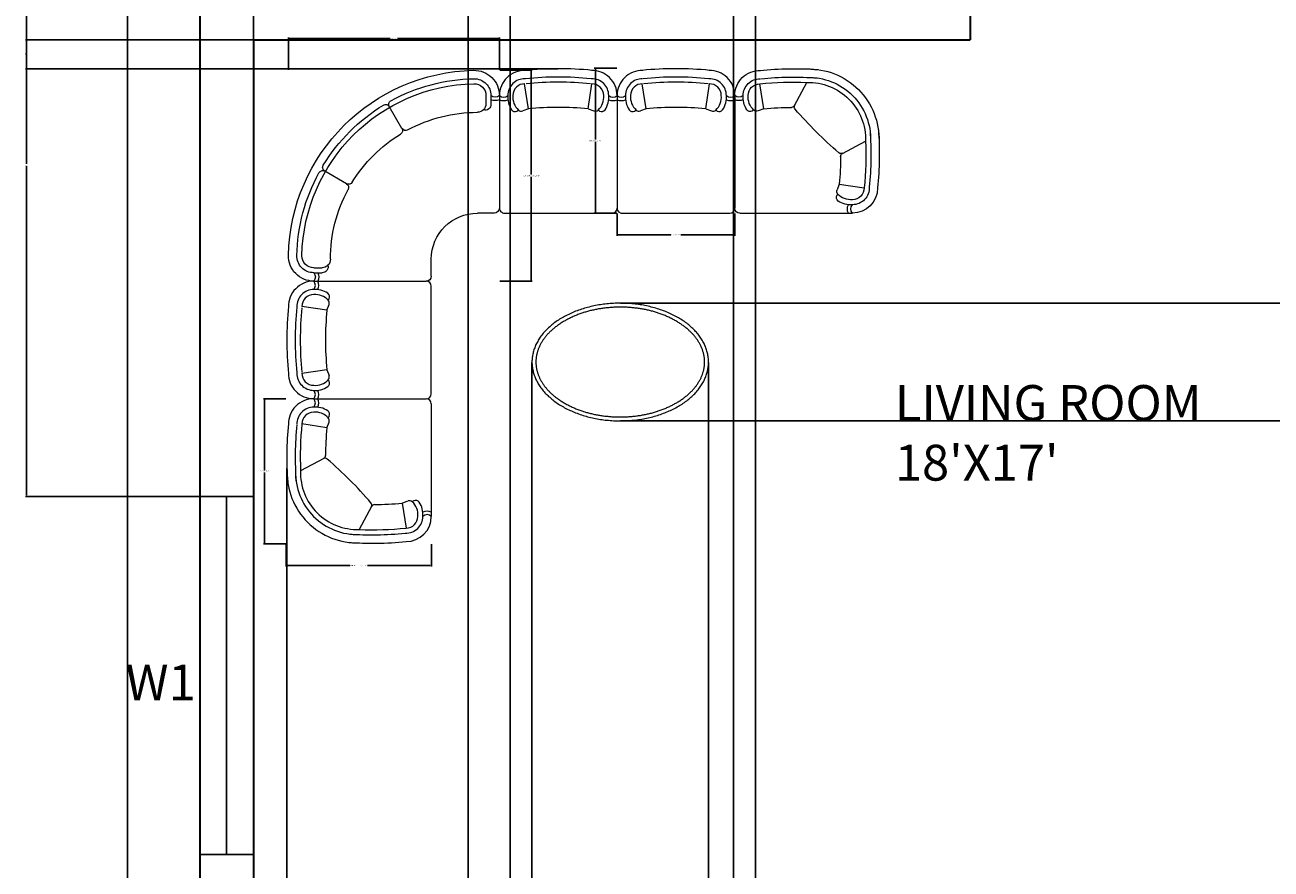
# Model space of a CAD drawing. Units: inches. Extents: x 3 to 420, y -502 to 54.
# Tile 2 of 6: x 3 to 212, y -398 to -257. Entities that reach past the tile are written whole.
import ezdxf

# ---------------------------------------------------------------- set-up
doc = ezdxf.new("R2010")
doc.units = ezdxf.units.IN
doc.header["$MEASUREMENT"] = 0
for name, color, linetype, lineweight in [('A-ANNO-DIMS', 2, 'Continuous', 18), ('A-ANNO-TEXT', 7, 'Continuous', 18), ('A-AREA-IDEN', 7, 'Continuous', 18), ('A-FURN', 8, 'Continuous', 18), ('A-GLAZ', 40, 'Continuous', 25), ('A-WALL', 7, 'Continuous', 35)]:
    doc.layers.add(name, color=color, linetype=linetype, lineweight=lineweight)
doc.styles.get("Standard").update_dxf_attribs({"font": 'arial.ttf'})
doc.dimstyles.get("Standard").update_dxf_attribs({"dimtxt": 0.18, "dimasz": 0.18, "dimexe": 0.18, "dimexo": 0.0625, "dimgap": 0.09, "dimtad": 0, "dimtih": 1, "dimtoh": 1, "dimdec": 0, "dimzin": 0, "dimdsep": 46, "dimlunit": 3, "dimtxsty": 'Standard', "dimcen": 0.09, "dimadec": 0, "dimazin": 0, "dimtfac": 1, "dimtdec": 0, "dimtofl": 0, "dimtmove": 0, "dimatfit": 3, "dimfxl": 1, "dimtolj": 1, "dimtzin": 0, "dimarcsym": 0})

# ---------------------------------------------------------------- blocks, each defined once
blk = doc.blocks.new('*D2')
at = {"layer": 'A-ANNO-DIMS', "color": 0, "lineweight": -2, "transparency": 16777216}
for p, q in [((32.33, 4.54), (20.1, 4.54)), ((20.28, 4.36), (20.28, -230.8)), ((20.28, -472.28), (20.28, -237.11)), ((32.33, -472.46), (20.1, -472.46))]:
    blk.add_line(p, q, dxfattribs=at)
at = {"layer": 'A-ANNO-DIMS', "color": 0, "transparency": 16777216}
for points in [[(20.25, 4.36), (20.31, 4.36), (20.28, 4.54)], [(20.25, -472.28), (20.31, -472.28), (20.28, -472.46)]]:
    blk.add_solid(points, dxfattribs=at)
at = {"layer": 'Defpoints', "color": 0, "transparency": 16777216}
for p in [(32.39, 4.54), (20.28, -472.46), (32.39, -472.46)]:
    blk.add_point(p, dxfattribs=at)
at = {"layer": 'A-ANNO-DIMS', "color": 0, "transparency": 16777216, "insert": (20.28, -233.96), "char_height": 6, "attachment_point": 5}
blk.add_mtext('\\A1;39\'-9"', dxfattribs=at)
blk = doc.blocks.new('A$C707258B2')
at = {"color": 0}
for p, q in [((0.4042, 0.342), (1.0739, 0.342)), ((1.1039, 0.312), (1.1039, 0.212)), ((0.4042, 0.292), (0.4544, 0.292)), ((0.4042, 0.262), (0.4539, 0.262)), ((1.4789, -0.063), (1.3789, -0.063)), ((1.5089, -0.7628), (1.5089, -0.093)), ((0.5998, -0.2378), (0.4699, -0.3128)), ((0.9291, -0.5671), (0.8541, -0.697)), ((1.4289, -0.7628), (1.4289, -0.713)), ((1.4589, -0.7628), (1.4589, -0.7125))]:
    blk.add_line(p, q, dxfattribs=at)
for centre, radius, start, end in [((0.4042, 0.192), 0.15, 90, 181.17538), ((0.3779, 0.317), 0.0362, 316.39718, 43.60282), ((0.3679, 0.317), 0.0662, 337.82984, 22.17016), ((1.0739, 0.312), 0.03, 360, 90), ((0.4042, 0.192), 0.1, 90, 181.17538), ((0.4042, 0.192), 0.07, 90, 181.17538), ((0.4539, 0.212), 0.05, 360, 90), ((0.4548, 0.2564), 0.0357, 345.42616, 90.55549), ((1.3789, 0.212), 1.125, 181.17538, 268.82462), ((1.3789, 0.212), 1.075, 181.17538, 208.63569), ((1.3789, 0.212), 1.045, 181.17538, 268.82462), ((1.3789, 0.212), 0.875, 180, 208.40825), ((1.3789, 0.212), 0.275, 180, 270), ((1.4789, -0.093), 0.03, 360, 90), ((0.5873, -0.2162), 0.025, 300, 28.40825), ((0.6123, -0.2595), 0.025, 31.59175, 120), ((1.3789, 0.212), 0.875, 211.59175, 238.40825), ((0.4574, -0.2912), 0.025, 208.63569, 300), ((0.4824, -0.3345), 0.025, 120, 211.36431), ((1.3789, 0.212), 1.075, 211.36431, 238.63569), ((0.9075, -0.5546), 0.025, 330, 58.40825), ((0.9508, -0.5796), 0.025, 61.59175, 150), ((1.3789, 0.212), 0.875, 241.59175, 270), ((1.3789, -0.713), 0.05, 360, 90), ((0.8324, -0.6845), 0.025, 238.63569, 330), ((0.8757, -0.7095), 0.025, 150, 241.36431), ((1.3789, 0.212), 1.075, 241.36431, 268.82462), ((1.4255, -0.7093), 0.0336, 354.63008, 109.38826), ((1.4839, -0.7988), 0.0662, 67.82984, 112.17016), ((1.3589, -0.7628), 0.15, 268.82462, 360), ((1.3589, -0.7628), 0.1, 268.82462, 360), ((1.3589, -0.7628), 0.07, 268.82462, 360), ((1.4839, -0.789), 0.0362, 46.39718, 133.60282)]:
    blk.add_arc(centre, radius, start, end, dxfattribs=at)
blk = doc.blocks.new('part 01')
at = {"color": 0}
for p, q in [((-669.8, 700), (0, 700)), ((30, 30), (30, 670)), ((-590.9, 527.1), (-739.8, 550)), ((-590.9, 527.1), (-578.5, 561.2)), ((-590.9, 172.9), (-739.8, 150)), ((-590.9, 172.9), (-578.5, 138.8)), ((-669.8, 0), (0, 0))]:
    blk.add_line(p, q, dxfattribs=at)
for centre, radius, start, end in [((-669.8, 550), 150, 90, 181.17538), ((-696, 675), 36.2, 316.39718, 43.60282), ((-705.9, 675), 66.2, 337.82984, 22.17016), ((0, 670), 30, 0, 90), ((-669.8, 550), 100, 90, 181.17538), ((-669.8, 550), 70, 90, 181.17538), ((-659.7, 517.8), 132.7, 56.08973, 95.61316), ((-659.7, 517.8), 102.7, 42.00663, 95.61316), ((-599.7, 607.2), 25, 332.96082, 56.08973), ((-624.8, 620), 53.2, 321.00172, 332.96082), ((1178.1, 350), 2007.9, 174.28354, 185.71646), ((1178.1, 350), 1957.9, 174.28354, 185.71646), ((1178.1, 350), 1927.9, 174.28354, 185.71646), ((1178.1, 350), 1777.9, 174.28354, 185.71646), ((-602, 569.8), 25, 340, 42.00663), ((-669.8, 150), 150, 178.82462, 270), ((-669.8, 150), 100, 178.82462, 270), ((-669.8, 150), 70, 178.82462, 270), ((-659.7, 182.2), 102.7, 264.38684, 317.99337), ((-599.7, 92.8), 25, 303.91027, 27.03918), ((-602, 130.2), 25, 317.99337, 20), ((-624.8, 80), 53.2, 27.03918, 38.99828), ((-659.7, 182.2), 132.7, 264.38684, 303.91027), ((-696, 25), 36.2, 316.39718, 43.60282), ((-705.9, 25), 66.2, 337.82984, 22.17016), ((0, 30), 30, 270, 0)]:
    blk.add_arc(centre, radius, start, end, dxfattribs=at)
blk = doc.blocks.new('part02')
at = {"color": 0}
for p, q in [((0, -669.8), (0, 0)), ((30, 30), (699.8, 30)), ((620.9, -142.9), (608.5, -108.8)), ((620.9, -142.9), (769.8, -120)), ((640.4, -325.6), (778.2, -398.9)), ((172.9, -590.9), (138.8, -578.5)), ((172.9, -590.9), (150, -739.8)), ((355.6, -610.4), (428.9, -748.2))]:
    blk.add_line(p, q, dxfattribs=at)
for centre, radius, start, end in [((30, 0), 30, 90, 180), ((726, 5), 56.2, 153.6122, 206.66656), ((726, 5), 36.2, 136.39718, 223.60282), ((699.8, -120), 150, 0, 90), ((629.7, -62.8), 25, 123.91027, 207.03918), ((689.7, -152.2), 102.7, 84.38684, 137.99337), ((689.3, -151.3), 131.7, 85.43775, 123.98866), ((699.5, -120.6), 100.6, 357.50055, 89.85796), ((699.8, -120), 70, 0, 90), ((632, -100.2), 25, 137.99337, 200), ((654.8, -50), 53.2, 207.03918, 218.99828), ((-1148.1, -320), 1777.9, 0.38365, 5.71646), ((-1228.2, -319.5), 2007.9, 357.73494, 5.70316), ((-1148.1, -320), 1957.9, 355.86566, 5.71646), ((-1148.1, -320), 2007.9, 355.81801, 5.71646), ((2219.8, -2189.8), 2454.4, 130.6961, 139.3039), ((632.4, -344.1), 20, 62, 130.6961), ((649.7, -308), 20, 180.38365, 242), ((439.4, -409.4), 418.9, 268.21809, 1.78191), ((439.4, -409.4), 368.9, 268.21809, 1.78191), ((439.4, -409.4), 338.9, 268.21809, 1.78191), ((182.2, -659.7), 132.7, 146.08973, 185.61316), ((92.8, -599.7), 25, 62.96082, 146.08973), ((182.2, -659.7), 102.7, 132.00663, 185.61316), ((80, -624.8), 53.2, 51.00172, 62.96082), ((130.2, -602), 25, 70, 132.00663), ((350, 1178.1), 1777.9, 264.28354, 269.61635), ((374.1, -602.4), 20, 139.3039, 208), ((25, -696), 56.2, 63.33344, 116.3878), ((25, -696), 36.2, 46.39718, 133.60282), ((338, -619.7), 20, 28, 89.61635), ((150, -669.8), 150, 180, 271.17538), ((150, -669.8), 100, 180, 271.17538), ((150, -669.8), 70, 180, 270), ((349.5, 1258.2), 2007.9, 264.29684, 272.26506), ((350, 1178.1), 1957.9, 264.28354, 274.13434), ((350, 1178.1), 2007.9, 264.28354, 274.18199)]:
    blk.add_arc(centre, radius, start, end, dxfattribs=at)
blk = doc.blocks.new('WIN-W1-60')
for p, q in [((0, 9), (60, 9)), ((0, 9), (0, 0)), ((60, 9), (60, 0)), ((0, 4.5), (60, 4.5)), ((0, 0), (60, 0))]:
    blk.add_line(p, q)
blk = doc.blocks.new('*D21')
at = {"layer": 'A-ANNO-DIMS', "color": 0, "lineweight": -2, "transparency": 16777216}
for p, q in [((102.21, -264.22), (98.45, -264.22)), ((98.63, -264.4), (98.63, -276.18)), ((98.63, -288.33), (98.63, -276.55)), ((102.21, -288.51), (98.45, -288.51))]:
    blk.add_line(p, q, dxfattribs=at)
at = {"layer": 'A-ANNO-DIMS', "color": 0, "transparency": 16777216}
for points in [[(98.6, -264.4), (98.66, -264.4), (98.63, -264.22)], [(98.6, -288.33), (98.66, -288.33), (98.63, -288.51)]]:
    blk.add_solid(points, dxfattribs=at)
at = {"layer": 'Defpoints', "color": 0, "transparency": 16777216}
for p in [(102.27, -264.22), (98.63, -288.51), (102.27, -288.51)]:
    blk.add_point(p, dxfattribs=at)
at = {"layer": 'A-ANNO-DIMS', "color": 0, "transparency": 16777216, "insert": (98.63, -276.37), "char_height": 0.18, "attachment_point": 5}
blk.add_mtext('\\A1;SEAT 2\'-0 1/2" TYP.', dxfattribs=at)
blk = doc.blocks.new('*D22')
at = {"layer": 'A-ANNO-DIMS', "color": 0, "lineweight": -2, "transparency": 16777216}
for p, q in [((102.27, -288.57), (102.27, -292.34)), ((121.97, -288.57), (121.97, -292.34)), ((102.45, -292.16), (111.28, -292.16)), ((121.79, -292.16), (112.96, -292.16))]:
    blk.add_line(p, q, dxfattribs=at)
at = {"layer": 'A-ANNO-DIMS', "color": 0, "transparency": 16777216}
for points in [[(102.45, -292.13), (102.45, -292.19), (102.27, -292.16)], [(121.79, -292.13), (121.79, -292.19), (121.97, -292.16)]]:
    blk.add_solid(points, dxfattribs=at)
at = {"layer": 'Defpoints', "color": 0, "transparency": 16777216}
for p in [(102.27, -288.51), (121.97, -288.51), (121.97, -292.16)]:
    blk.add_point(p, dxfattribs=at)
at = {"layer": 'A-ANNO-DIMS', "color": 0, "transparency": 16777216, "insert": (112.12, -292.16), "char_height": 0.18, "attachment_point": 5}
blk.add_mtext('\\A1;1\'-7 1/2" TYP.', dxfattribs=at)
blk = doc.blocks.new('*D23')
at = {"layer": 'A-ANNO-DIMS', "color": 0, "lineweight": -2, "transparency": 16777216}
for p, q in [((46.88, -343.96), (46.88, -347.72)), ((71.17, -343.96), (71.17, -347.72)), ((47.06, -347.54), (57.55, -347.54)), ((70.99, -347.54), (60.5, -347.54))]:
    blk.add_line(p, q, dxfattribs=at)
at = {"layer": 'A-ANNO-DIMS', "color": 0, "transparency": 16777216}
for points in [[(47.06, -347.51), (47.06, -347.57), (46.88, -347.54)], [(70.99, -347.51), (70.99, -347.57), (71.17, -347.54)]]:
    blk.add_solid(points, dxfattribs=at)
at = {"layer": 'Defpoints', "color": 0, "transparency": 16777216}
for p in [(46.88, -343.9), (71.17, -343.9), (71.17, -347.54)]:
    blk.add_point(p, dxfattribs=at)
at = {"layer": 'A-ANNO-DIMS', "color": 0, "transparency": 16777216, "insert": (59.02, -347.54), "char_height": 0.18, "attachment_point": 5}
blk.add_mtext('\\A1;END UNIT 2\'-0 1/2" TYP.', dxfattribs=at)
blk = doc.blocks.new('*D24')
at = {"layer": 'A-ANNO-DIMS', "color": 0, "lineweight": -2, "transparency": 16777216}
for p, q in [((46.82, -319.61), (43.06, -319.61)), ((43.24, -319.79), (43.24, -331.57)), ((43.24, -343.72), (43.24, -331.94)), ((46.82, -343.9), (43.06, -343.9))]:
    blk.add_line(p, q, dxfattribs=at)
at = {"layer": 'A-ANNO-DIMS', "color": 0, "transparency": 16777216}
for points in [[(43.21, -319.79), (43.27, -319.79), (43.24, -319.61)], [(43.21, -343.72), (43.27, -343.72), (43.24, -343.9)]]:
    blk.add_solid(points, dxfattribs=at)
at = {"layer": 'Defpoints', "color": 0, "transparency": 16777216}
for p in [(46.88, -319.61), (43.24, -343.9), (46.88, -343.9)]:
    blk.add_point(p, dxfattribs=at)
at = {"layer": 'A-ANNO-DIMS', "color": 0, "transparency": 16777216, "insert": (43.24, -331.76), "char_height": 0.18, "attachment_point": 5}
blk.add_mtext('\\A1;2\'-0 1/2" TYP.', dxfattribs=at)
blk = doc.blocks.new('*D25')
at = {"layer": 'A-ANNO-DIMS', "color": 0, "lineweight": -2, "transparency": 16777216}
for p, q in [((82.63, -264.57), (88.05, -264.57)), ((87.87, -264.75), (87.87, -282.06)), ((87.87, -299.73), (87.87, -282.42)), ((82.63, -299.91), (88.05, -299.91))]:
    blk.add_line(p, q, dxfattribs=at)
at = {"layer": 'A-ANNO-DIMS', "color": 0, "transparency": 16777216}
for points in [[(87.84, -264.75), (87.9, -264.75), (87.87, -264.57)], [(87.84, -299.73), (87.9, -299.73), (87.87, -299.91)]]:
    blk.add_solid(points, dxfattribs=at)
at = {"layer": 'Defpoints', "color": 0, "transparency": 16777216}
for p in [(82.57, -264.57), (82.57, -299.91), (87.87, -299.91)]:
    blk.add_point(p, dxfattribs=at)
at = {"layer": 'A-ANNO-DIMS', "color": 0, "transparency": 16777216, "insert": (87.87, -282.24), "char_height": 0.18, "attachment_point": 5}
blk.add_mtext('\\A1;CORNER UNIT 2\'-11 1/2"', dxfattribs=at)
blk = doc.blocks.new('*D26')
at = {"layer": 'A-ANNO-DIMS', "color": 0, "lineweight": -2, "transparency": 16777216}
for p, q in [((47.23, -264.51), (47.23, -259.09)), ((47.41, -259.27), (64.29, -259.27)), ((82.39, -259.27), (65.51, -259.27)), ((82.57, -264.51), (82.57, -259.09))]:
    blk.add_line(p, q, dxfattribs=at)
at = {"layer": 'A-ANNO-DIMS', "color": 0, "transparency": 16777216}
for points in [[(47.41, -259.24), (47.41, -259.3), (47.23, -259.27)], [(82.39, -259.24), (82.39, -259.3), (82.57, -259.27)]]:
    blk.add_solid(points, dxfattribs=at)
at = {"layer": 'Defpoints', "color": 0, "transparency": 16777216}
for p in [(82.57, -259.27), (47.23, -264.57), (82.57, -264.57)]:
    blk.add_point(p, dxfattribs=at)
at = {"layer": 'A-ANNO-DIMS', "color": 0, "transparency": 16777216, "insert": (64.9, -259.27), "char_height": 0.18, "attachment_point": 5}
blk.add_mtext('\\A1;2\'-11 1/2"', dxfattribs=at)
blk = doc.blocks.new('*D39')
at = {"layer": 'A-ANNO-DIMS', "color": 0, "lineweight": -2, "transparency": 16777216}
for p, q in [((41.39, -130.52), (41.39, -501.64)), ((77.36, -130.52), (77.36, -501.64)), ((41.57, -501.46), (59.04, -501.46)), ((77.18, -501.46), (59.7, -501.46))]:
    blk.add_line(p, q, dxfattribs=at)
at = {"layer": 'A-ANNO-DIMS', "color": 0, "transparency": 16777216}
for points in [[(41.57, -501.43), (41.57, -501.49), (41.39, -501.46)], [(77.18, -501.43), (77.18, -501.49), (77.36, -501.46)]]:
    blk.add_solid(points, dxfattribs=at)
at = {"layer": 'Defpoints', "color": 0, "transparency": 16777216}
for p in [(41.39, -130.46), (77.36, -130.46), (77.36, -501.46)]:
    blk.add_point(p, dxfattribs=at)
at = {"layer": 'A-ANNO-DIMS', "color": 0, "transparency": 16777216, "insert": (59.37, -501.46), "char_height": 0.18, "attachment_point": 5}
blk.add_mtext('\\A1;3\'-0"', dxfattribs=at)
blk = doc.blocks.new('*D46')
at = {"layer": 'A-ANNO-DIMS', "color": 0, "lineweight": -2, "transparency": 16777216}
for p, q in [((41.39, -135.02), (41.39, -501.64)), ((121.75, -135.02), (121.75, -501.64)), ((41.57, -501.46), (81.03, -501.46)), ((121.57, -501.46), (82.11, -501.46))]:
    blk.add_line(p, q, dxfattribs=at)
at = {"layer": 'A-ANNO-DIMS', "color": 0, "transparency": 16777216}
for points in [[(41.57, -501.43), (41.57, -501.49), (41.39, -501.46)], [(121.57, -501.43), (121.57, -501.49), (121.75, -501.46)]]:
    blk.add_solid(points, dxfattribs=at)
at = {"layer": 'Defpoints', "color": 0, "transparency": 16777216}
for p in [(41.39, -134.96), (121.75, -134.96), (121.75, -501.46)]:
    blk.add_point(p, dxfattribs=at)
at = {"layer": 'A-ANNO-DIMS', "color": 0, "transparency": 16777216, "insert": (81.57, -501.46), "char_height": 0.18, "attachment_point": 5}
blk.add_mtext('\\A1;6\'-8 1/2"', dxfattribs=at)
blk = doc.blocks.new('*D61')
at = {"layer": 'A-ANNO-DIMS', "color": 0, "lineweight": -2, "transparency": 16777216}
for p, q in [((32.33, -224.96), (3.21, -224.96)), ((3.39, -225.14), (3.39, -280.27)), ((3.39, -335.78), (3.39, -280.64)), ((32.33, -335.96), (3.21, -335.96))]:
    blk.add_line(p, q, dxfattribs=at)
at = {"layer": 'A-ANNO-DIMS', "color": 0, "transparency": 16777216}
for points in [[(3.36, -225.14), (3.42, -225.14), (3.39, -224.96)], [(3.36, -335.78), (3.42, -335.78), (3.39, -335.96)]]:
    blk.add_solid(points, dxfattribs=at)
at = {"layer": 'Defpoints', "color": 0, "transparency": 16777216}
for p in [(32.39, -224.96), (3.39, -335.96), (32.39, -335.96)]:
    blk.add_point(p, dxfattribs=at)
at = {"layer": 'A-ANNO-DIMS', "color": 0, "transparency": 16777216, "insert": (3.39, -280.46), "char_height": 0.18, "attachment_point": 5}
blk.add_mtext('\\A1;9\'-3"', dxfattribs=at)
blk = doc.blocks.new('*D62')
at = {"layer": 'A-ANNO-DIMS', "color": 0, "lineweight": -2, "transparency": 16777216}
for p, q in [((84.39, -463.39), (84.39, 33.72)), ((84.57, 33.54), (104.58, 33.54)), ((125.25, 33.54), (105.24, 33.54)), ((125.43, -463.39), (125.43, 33.72))]:
    blk.add_line(p, q, dxfattribs=at)
at = {"layer": 'A-ANNO-DIMS', "color": 0, "transparency": 16777216}
for points in [[(84.57, 33.57), (84.57, 33.51), (84.39, 33.54)], [(125.25, 33.57), (125.25, 33.51), (125.43, 33.54)]]:
    blk.add_solid(points, dxfattribs=at)
at = {"layer": 'Defpoints', "color": 0, "transparency": 16777216}
for p in [(125.43, 33.54), (84.39, -463.46), (125.43, -463.46)]:
    blk.add_point(p, dxfattribs=at)
at = {"layer": 'A-ANNO-DIMS', "color": 0, "transparency": 16777216, "insert": (104.91, 33.54), "char_height": 0.18, "attachment_point": 5}
blk.add_mtext('\\A1;3\'-5"', dxfattribs=at)
blk = doc.blocks.new('*D73')
at = {"layer": 'A-ANNO-DIMS', "color": 0, "lineweight": -2, "transparency": 16777216}
for p, q in [((88.02, -313.52), (88.02, -501.64)), ((117.58, -313.52), (117.58, -501.64)), ((88.2, -501.46), (102.26, -501.46)), ((117.4, -501.46), (103.34, -501.46))]:
    blk.add_line(p, q, dxfattribs=at)
at = {"layer": 'A-ANNO-DIMS', "color": 0, "transparency": 16777216}
for points in [[(88.2, -501.43), (88.2, -501.49), (88.02, -501.46)], [(117.4, -501.43), (117.4, -501.49), (117.58, -501.46)]]:
    blk.add_solid(points, dxfattribs=at)
at = {"layer": 'Defpoints', "color": 0, "transparency": 16777216}
for p in [(88.02, -313.46), (117.58, -313.46), (117.58, -501.46)]:
    blk.add_point(p, dxfattribs=at)
at = {"layer": 'A-ANNO-DIMS', "color": 0, "transparency": 16777216, "insert": (102.8, -501.46), "char_height": 0.18, "attachment_point": 5}
blk.add_mtext('\\A1;2\'-5 1/2"', dxfattribs=at)
blk = doc.blocks.new('*D74')
at = {"layer": 'A-ANNO-DIMS', "color": 0, "lineweight": -2, "transparency": 16777216}
for p, q in [((102.86, -303.61), (420.07, -303.61)), ((419.89, -303.79), (419.89, -313.28)), ((419.89, -323.13), (419.89, -313.64)), ((102.86, -323.31), (420.07, -323.31))]:
    blk.add_line(p, q, dxfattribs=at)
at = {"layer": 'A-ANNO-DIMS', "color": 0, "transparency": 16777216}
for points in [[(419.86, -303.79), (419.92, -303.79), (419.89, -303.61)], [(419.86, -323.13), (419.92, -323.13), (419.89, -323.31)]]:
    blk.add_solid(points, dxfattribs=at)
at = {"layer": 'Defpoints', "color": 0, "transparency": 16777216}
for p in [(102.8, -303.61), (102.8, -323.31), (419.89, -323.31)]:
    blk.add_point(p, dxfattribs=at)
at = {"layer": 'A-ANNO-DIMS', "color": 0, "transparency": 16777216, "insert": (419.89, -313.46), "char_height": 0.18, "attachment_point": 5}
blk.add_mtext('\\A1;1\'-7 1/2"', dxfattribs=at)
blk = doc.blocks.new('*D78')
at = {"layer": 'A-ANNO-DIMS', "color": 0, "lineweight": -2, "transparency": 16777216}
for p, q in [((46.99, -331.21), (46.99, -501.64)), ((41.39, -336.02), (41.39, -501.64)), ((41.57, -501.46), (43.65, -501.46)), ((46.81, -501.46), (44.73, -501.46))]:
    blk.add_line(p, q, dxfattribs=at)
at = {"layer": 'A-ANNO-DIMS', "color": 0, "transparency": 16777216}
for points in [[(41.57, -501.43), (41.57, -501.49), (41.39, -501.46)], [(46.81, -501.43), (46.81, -501.49), (46.99, -501.46)]]:
    blk.add_solid(points, dxfattribs=at)
at = {"layer": 'Defpoints', "color": 0, "transparency": 16777216}
for p in [(46.99, -331.15), (41.39, -335.96), (46.99, -501.46)]:
    blk.add_point(p, dxfattribs=at)
at = {"layer": 'A-ANNO-DIMS', "color": 0, "transparency": 16777216, "insert": (44.19, -501.46), "char_height": 0.18, "attachment_point": 5}
blk.add_mtext('\\A1;0\'-5 1/2"', dxfattribs=at)
blk = doc.blocks.new('*D79')
at = {"layer": 'A-ANNO-DIMS', "color": 0, "lineweight": -2, "transparency": 16777216}
for p, q in [((41.33, -259.46), (3.21, -259.46)), ((3.39, -259.64), (3.39, -261.7)), ((3.39, -264.13), (3.39, -262.07)), ((92.36, -264.31), (3.21, -264.31))]:
    blk.add_line(p, q, dxfattribs=at)
at = {"layer": 'A-ANNO-DIMS', "color": 0, "transparency": 16777216}
for points in [[(3.36, -259.64), (3.42, -259.64), (3.39, -259.46)], [(3.36, -264.13), (3.42, -264.13), (3.39, -264.31)]]:
    blk.add_solid(points, dxfattribs=at)
at = {"layer": 'Defpoints', "color": 0, "transparency": 16777216}
for p in [(41.39, -259.46), (3.39, -264.31), (92.42, -264.31)]:
    blk.add_point(p, dxfattribs=at)
at = {"layer": 'A-ANNO-DIMS', "color": 0, "transparency": 16777216, "insert": (3.39, -261.88), "char_height": 0.18, "attachment_point": 5}
blk.add_mtext('\\A1;0\'-5"', dxfattribs=at)

msp = doc.modelspace()

# ---------------------------------------------------------------- linework, layer by layer
at = {"layer": 'A-FURN', "ltscale": 0.03}
msp.add_polyline3d([(117.58, -313.46, 0), (117.57, -313.27, 0), (117.57, -313.09, 0), (117.55, -312.9, 0), (117.53, -312.71, 0), (117.51, -312.53, 0), (117.48, -312.34, 0), (117.45, -312.16, 0), (117.41, -311.97, 0), (117.36, -311.79, 0), (117.31, -311.61, 0), (117.26, -311.42, 0), (117.2, -311.24, 0), (117.13, -311.06, 0), (117.06, -310.88, 0), (116.98, -310.7, 0), (116.9, -310.52, 0), (116.82, -310.34, 0), (116.73, -310.17, 0), (116.63, -309.99, 0), (116.53, -309.82, 0), (116.42, -309.65, 0), (116.31, -309.47, 0), (116.2, -309.3, 0), (116.08, -309.14, 0), (115.95, -308.97, 0), (115.82, -308.8, 0), (115.69, -308.64, 0), (115.55, -308.48, 0), (115.41, -308.32, 0), (115.26, -308.16, 0), (115.11, -308.01, 0), (114.95, -307.85, 0), (114.79, -307.7, 0), (114.62, -307.55, 0), (114.45, -307.4, 0), (114.28, -307.25, 0), (114.1, -307.11, 0), (113.92, -306.97, 0), (113.73, -306.83, 0), (113.54, -306.69, 0), (113.35, -306.56, 0), (113.15, -306.43, 0), (112.95, -306.3, 0), (112.74, -306.17, 0), (112.53, -306.05, 0), (112.32, -305.93, 0), (112.11, -305.81, 0), (111.89, -305.69, 0), (111.66, -305.58, 0), (111.44, -305.47, 0), (111.21, -305.36, 0), (110.98, -305.25, 0), (110.75, -305.15, 0), (110.51, -305.05, 0), (110.27, -304.96, 0), (110.03, -304.87, 0), (109.78, -304.78, 0), (109.53, -304.69, 0), (109.28, -304.61, 0), (109.03, -304.53, 0), (108.78, -304.45, 0), (108.52, -304.38, 0), (108.26, -304.3, 0), (108, -304.24, 0), (107.74, -304.17, 0), (107.47, -304.11, 0), (107.21, -304.06, 0), (106.94, -304, 0), (106.67, -303.95, 0), (106.4, -303.9, 0), (106.13, -303.86, 0), (105.85, -303.82, 0), (105.58, -303.78, 0), (105.3, -303.75, 0), (105.03, -303.72, 0), (104.75, -303.69, 0), (104.47, -303.67, 0), (104.2, -303.65, 0), (103.92, -303.64, 0), (103.64, -303.62, 0), (103.36, -303.61, 0), (103.08, -303.61, 0), (102.8, -303.61, 0), (102.52, -303.61, 0), (102.24, -303.61, 0), (101.96, -303.62, 0), (101.68, -303.64, 0), (101.4, -303.65, 0), (101.12, -303.67, 0), (100.85, -303.69, 0), (100.57, -303.72, 0), (100.29, -303.75, 0), (100.02, -303.78, 0), (99.75, -303.82, 0), (99.47, -303.86, 0), (99.2, -303.9, 0), (98.93, -303.95, 0), (98.66, -304, 0), (98.39, -304.06, 0), (98.13, -304.11, 0), (97.86, -304.17, 0), (97.6, -304.24, 0), (97.34, -304.3, 0), (97.08, -304.38, 0), (96.82, -304.45, 0), (96.57, -304.53, 0), (96.32, -304.61, 0), (96.07, -304.69, 0), (95.82, -304.78, 0), (95.57, -304.87, 0), (95.33, -304.96, 0), (95.09, -305.05, 0), (94.85, -305.15, 0), (94.62, -305.25, 0), (94.39, -305.36, 0), (94.16, -305.47, 0), (93.93, -305.58, 0), (93.71, -305.69, 0), (93.49, -305.81, 0), (93.28, -305.93, 0), (93.06, -306.05, 0), (92.86, -306.17, 0), (92.65, -306.3, 0), (92.45, -306.43, 0), (92.25, -306.56, 0), (92.06, -306.69, 0), (91.87, -306.83, 0), (91.68, -306.97, 0), (91.5, -307.11, 0), (91.32, -307.25, 0), (91.15, -307.4, 0), (90.98, -307.55, 0), (90.81, -307.7, 0), (90.65, -307.85, 0), (90.49, -308.01, 0), (90.34, -308.16, 0), (90.19, -308.32, 0), (90.05, -308.48, 0), (89.91, -308.64, 0), (89.78, -308.8, 0), (89.65, -308.97, 0), (89.52, -309.14, 0), (89.4, -309.3, 0), (89.28, -309.47, 0), (89.17, -309.65, 0), (89.07, -309.82, 0), (88.97, -309.99, 0), (88.87, -310.17, 0), (88.78, -310.34, 0), (88.69, -310.52, 0), (88.61, -310.7, 0), (88.54, -310.88, 0), (88.47, -311.06, 0), (88.4, -311.24, 0), (88.34, -311.42, 0), (88.29, -311.61, 0), (88.24, -311.79, 0), (88.19, -311.97, 0), (88.15, -312.16, 0), (88.12, -312.34, 0), (88.09, -312.53, 0), (88.06, -312.71, 0), (88.05, -312.9, 0), (88.03, -313.09, 0), (88.02, -313.27, 0), (88.02, -313.46, 0), (88.02, -313.65, 0), (88.03, -313.83, 0), (88.05, -314.02, 0), (88.06, -314.2, 0), (88.09, -314.39, 0), (88.12, -314.57, 0), (88.15, -314.76, 0), (88.19, -314.94, 0), (88.24, -315.13, 0), (88.29, -315.31, 0), (88.34, -315.49, 0), (88.4, -315.68, 0), (88.47, -315.86, 0), (88.54, -316.04, 0), (88.61, -316.22, 0), (88.69, -316.4, 0), (88.78, -316.57, 0), (88.87, -316.75, 0), (88.97, -316.93, 0), (89.07, -317.1, 0), (89.17, -317.27, 0), (89.28, -317.44, 0), (89.4, -317.61, 0), (89.52, -317.78, 0), (89.65, -317.95, 0), (89.78, -318.11, 0), (89.91, -318.28, 0), (90.05, -318.44, 0), (90.19, -318.6, 0), (90.34, -318.76, 0), (90.49, -318.91, 0), (90.65, -319.07, 0), (90.81, -319.22, 0), (90.98, -319.37, 0), (91.15, -319.52, 0), (91.32, -319.66, 0), (91.5, -319.81, 0), (91.68, -319.95, 0), (91.87, -320.09, 0), (92.06, -320.22, 0), (92.25, -320.36, 0), (92.45, -320.49, 0), (92.65, -320.62, 0), (92.86, -320.75, 0), (93.06, -320.87, 0), (93.28, -320.99, 0), (93.49, -321.11, 0), (93.71, -321.23, 0), (93.93, -321.34, 0), (94.16, -321.45, 0), (94.39, -321.56, 0), (94.62, -321.66, 0), (94.85, -321.76, 0), (95.09, -321.86, 0), (95.33, -321.96, 0), (95.57, -322.05, 0), (95.82, -322.14, 0), (96.07, -322.23, 0), (96.32, -322.31, 0), (96.57, -322.39, 0), (96.82, -322.47, 0), (97.08, -322.54, 0), (97.34, -322.61, 0), (97.6, -322.68, 0), (97.86, -322.74, 0), (98.13, -322.8, 0), (98.39, -322.86, 0), (98.66, -322.92, 0), (98.93, -322.97, 0), (99.2, -323.01, 0), (99.47, -323.06, 0), (99.75, -323.1, 0), (100.02, -323.13, 0), (100.29, -323.17, 0), (100.57, -323.2, 0), (100.85, -323.22, 0), (101.12, -323.25, 0), (101.4, -323.27, 0), (101.68, -323.28, 0), (101.96, -323.29, 0), (102.24, -323.3, 0), (102.52, -323.31, 0), (102.8, -323.31, 0), (103.08, -323.31, 0), (103.36, -323.3, 0), (103.64, -323.29, 0), (103.92, -323.28, 0), (104.2, -323.27, 0), (104.47, -323.25, 0), (104.75, -323.22, 0), (105.03, -323.2, 0), (105.3, -323.17, 0), (105.58, -323.13, 0), (105.85, -323.1, 0), (106.13, -323.06, 0), (106.4, -323.01, 0), (106.67, -322.97, 0), (106.94, -322.92, 0), (107.21, -322.86, 0), (107.47, -322.8, 0), (107.74, -322.74, 0), (108, -322.68, 0), (108.26, -322.61, 0), (108.52, -322.54, 0), (108.78, -322.47, 0), (109.03, -322.39, 0), (109.28, -322.31, 0), (109.53, -322.23, 0), (109.78, -322.14, 0), (110.03, -322.05, 0), (110.27, -321.96, 0), (110.51, -321.86, 0), (110.75, -321.76, 0), (110.98, -321.66, 0), (111.21, -321.56, 0), (111.44, -321.45, 0), (111.66, -321.34, 0), (111.89, -321.23, 0), (112.11, -321.11, 0), (112.32, -320.99, 0), (112.53, -320.87, 0), (112.74, -320.75, 0), (112.95, -320.62, 0), (113.15, -320.49, 0), (113.35, -320.36, 0), (113.54, -320.22, 0), (113.73, -320.09, 0), (113.92, -319.95, 0), (114.1, -319.81, 0), (114.28, -319.66, 0), (114.45, -319.52, 0), (114.62, -319.37, 0), (114.79, -319.22, 0), (114.95, -319.07, 0), (115.11, -318.91, 0), (115.26, -318.76, 0), (115.41, -318.6, 0), (115.55, -318.44, 0), (115.69, -318.28, 0), (115.82, -318.11, 0), (115.95, -317.95, 0), (116.08, -317.78, 0), (116.2, -317.61, 0), (116.31, -317.44, 0), (116.42, -317.27, 0), (116.53, -317.1, 0), (116.63, -316.93, 0), (116.73, -316.75, 0), (116.82, -316.57, 0), (116.9, -316.4, 0), (116.98, -316.22, 0), (117.06, -316.04, 0), (117.13, -315.86, 0), (117.2, -315.68, 0), (117.26, -315.49, 0), (117.31, -315.31, 0), (117.36, -315.13, 0), (117.41, -314.94, 0), (117.45, -314.76, 0), (117.48, -314.57, 0), (117.51, -314.39, 0), (117.53, -314.2, 0), (117.55, -314.02, 0), (117.57, -313.83, 0), (117.57, -313.65, 0), (117.58, -313.46, 0)], dxfattribs=at)
at = {"layer": 'A-FURN'}
msp.add_polyline3d([(116.92, -313.46, 0), (116.92, -313.36, 0), (116.92, -313.26, 0), (116.91, -313.16, 0), (116.91, -313.05, 0), (116.9, -312.95, 0), (116.89, -312.85, 0), (116.88, -312.74, 0), (116.86, -312.64, 0), (116.85, -312.54, 0), (116.83, -312.43, 0), (116.81, -312.33, 0), (116.79, -312.22, 0), (116.77, -312.12, 0), (116.74, -312.01, 0), (116.71, -311.91, 0), (116.68, -311.8, 0), (116.65, -311.69, 0), (116.62, -311.59, 0), (116.58, -311.48, 0), (116.55, -311.37, 0), (116.51, -311.26, 0), (116.46, -311.16, 0), (116.42, -311.05, 0), (116.37, -310.94, 0), (116.32, -310.83, 0), (116.27, -310.73, 0), (116.22, -310.62, 0), (116.16, -310.51, 0), (116.11, -310.4, 0), (116.05, -310.29, 0), (115.98, -310.19, 0), (115.92, -310.08, 0), (115.85, -309.97, 0), (115.78, -309.86, 0), (115.71, -309.76, 0), (115.64, -309.65, 0), (115.56, -309.55, 0), (115.48, -309.44, 0), (115.4, -309.33, 0), (115.32, -309.23, 0), (115.24, -309.12, 0), (115.15, -309.02, 0), (115.06, -308.92, 0), (114.97, -308.81, 0), (114.87, -308.71, 0), (114.78, -308.61, 0), (114.68, -308.51, 0), (114.57, -308.41, 0), (114.47, -308.31, 0), (114.36, -308.21, 0), (114.26, -308.11, 0), (114.15, -308.01, 0), (114.03, -307.91, 0), (113.92, -307.82, 0), (113.8, -307.72, 0), (113.68, -307.63, 0), (113.56, -307.53, 0), (113.44, -307.44, 0), (113.31, -307.35, 0), (113.19, -307.26, 0), (113.06, -307.17, 0), (112.93, -307.08, 0), (112.79, -306.99, 0), (112.66, -306.9, 0), (112.52, -306.82, 0), (112.39, -306.73, 0), (112.25, -306.65, 0), (112.11, -306.57, 0), (111.96, -306.49, 0), (111.82, -306.41, 0), (111.67, -306.33, 0), (111.53, -306.25, 0), (111.38, -306.17, 0), (111.23, -306.1, 0), (111.08, -306.03, 0), (110.93, -305.95, 0), (110.77, -305.88, 0), (110.62, -305.81, 0), (110.46, -305.75, 0), (110.3, -305.68, 0), (110.14, -305.62, 0), (109.98, -305.55, 0), (109.82, -305.49, 0), (109.66, -305.43, 0), (109.5, -305.37, 0), (109.34, -305.32, 0), (109.17, -305.26, 0), (109.01, -305.21, 0), (108.84, -305.16, 0), (108.68, -305.1, 0), (108.51, -305.06, 0), (108.35, -305.01, 0), (108.18, -304.96, 0), (108.02, -304.92, 0), (107.85, -304.88, 0), (107.68, -304.83, 0), (107.52, -304.79, 0), (107.35, -304.76, 0), (107.18, -304.72, 0), (107.01, -304.68, 0), (106.85, -304.65, 0), (106.68, -304.62, 0), (106.51, -304.59, 0), (106.34, -304.56, 0), (106.17, -304.53, 0), (106, -304.5, 0), (105.83, -304.48, 0), (105.66, -304.45, 0), (105.49, -304.43, 0), (105.32, -304.41, 0), (105.15, -304.39, 0), (104.98, -304.37, 0), (104.81, -304.36, 0), (104.64, -304.34, 0), (104.47, -304.33, 0), (104.3, -304.32, 0), (104.13, -304.3, 0), (103.96, -304.29, 0), (103.78, -304.29, 0), (103.61, -304.28, 0), (103.44, -304.27, 0), (103.27, -304.27, 0), (103.1, -304.27, 0), (102.93, -304.26, 0), (102.76, -304.26, 0), (102.58, -304.27, 0), (102.41, -304.27, 0), (102.24, -304.27, 0), (102.07, -304.28, 0), (101.9, -304.28, 0), (101.73, -304.29, 0), (101.56, -304.3, 0), (101.39, -304.31, 0), (101.21, -304.32, 0), (101.04, -304.33, 0), (100.87, -304.35, 0), (100.7, -304.36, 0), (100.53, -304.38, 0), (100.36, -304.4, 0), (100.19, -304.42, 0), (100.02, -304.44, 0), (99.85, -304.47, 0), (99.68, -304.49, 0), (99.51, -304.52, 0), (99.34, -304.54, 0), (99.17, -304.57, 0), (99, -304.6, 0), (98.84, -304.63, 0), (98.67, -304.67, 0), (98.5, -304.7, 0), (98.33, -304.74, 0), (98.16, -304.77, 0), (98, -304.81, 0), (97.83, -304.85, 0), (97.66, -304.9, 0), (97.5, -304.94, 0), (97.33, -304.99, 0), (97.17, -305.03, 0), (97, -305.08, 0), (96.84, -305.13, 0), (96.67, -305.18, 0), (96.51, -305.23, 0), (96.34, -305.29, 0), (96.18, -305.34, 0), (96.02, -305.4, 0), (95.86, -305.46, 0), (95.69, -305.52, 0), (95.53, -305.58, 0), (95.37, -305.65, 0), (95.22, -305.71, 0), (95.06, -305.78, 0), (94.9, -305.85, 0), (94.75, -305.92, 0), (94.6, -305.99, 0), (94.44, -306.06, 0), (94.29, -306.14, 0), (94.14, -306.21, 0), (94, -306.29, 0), (93.85, -306.37, 0), (93.71, -306.45, 0), (93.56, -306.53, 0), (93.42, -306.61, 0), (93.28, -306.69, 0), (93.14, -306.78, 0), (93.01, -306.86, 0), (92.87, -306.95, 0), (92.74, -307.03, 0), (92.61, -307.12, 0), (92.48, -307.21, 0), (92.35, -307.3, 0), (92.22, -307.39, 0), (92.1, -307.49, 0), (91.98, -307.58, 0), (91.86, -307.67, 0), (91.74, -307.77, 0), (91.62, -307.87, 0), (91.51, -307.96, 0), (91.4, -308.06, 0), (91.29, -308.16, 0), (91.18, -308.26, 0), (91.08, -308.36, 0), (90.97, -308.46, 0), (90.87, -308.56, 0), (90.77, -308.66, 0), (90.68, -308.76, 0), (90.58, -308.87, 0), (90.49, -308.97, 0), (90.41, -309.07, 0), (90.32, -309.18, 0), (90.24, -309.28, 0), (90.15, -309.39, 0), (90.07, -309.49, 0), (90, -309.6, 0), (89.92, -309.7, 0), (89.85, -309.81, 0), (89.78, -309.92, 0), (89.71, -310.03, 0), (89.65, -310.13, 0), (89.58, -310.24, 0), (89.52, -310.35, 0), (89.46, -310.46, 0), (89.41, -310.56, 0), (89.35, -310.67, 0), (89.3, -310.78, 0), (89.25, -310.89, 0), (89.2, -310.99, 0), (89.16, -311.1, 0), (89.11, -311.21, 0), (89.07, -311.32, 0), (89.03, -311.43, 0), (89, -311.53, 0), (88.96, -311.64, 0), (88.93, -311.75, 0), (88.9, -311.85, 0), (88.87, -311.96, 0), (88.84, -312.06, 0), (88.82, -312.17, 0), (88.8, -312.27, 0), (88.78, -312.38, 0), (88.76, -312.48, 0), (88.74, -312.59, 0), (88.73, -312.69, 0), (88.72, -312.8, 0), (88.71, -312.9, 0), (88.7, -313, 0), (88.69, -313.1, 0), (88.68, -313.21, 0), (88.68, -313.31, 0), (88.68, -313.41, 0), (88.68, -313.51, 0), (88.68, -313.61, 0), (88.68, -313.71, 0), (88.69, -313.81, 0), (88.7, -313.92, 0), (88.71, -314.02, 0), (88.72, -314.12, 0), (88.73, -314.23, 0), (88.74, -314.33, 0), (88.76, -314.43, 0), (88.78, -314.54, 0), (88.8, -314.64, 0), (88.82, -314.75, 0), (88.84, -314.85, 0), (88.87, -314.96, 0), (88.9, -315.07, 0), (88.93, -315.17, 0), (88.96, -315.28, 0), (89, -315.39, 0), (89.03, -315.49, 0), (89.07, -315.6, 0), (89.11, -315.71, 0), (89.16, -315.81, 0), (89.2, -315.92, 0), (89.25, -316.03, 0), (89.3, -316.14, 0), (89.35, -316.25, 0), (89.41, -316.35, 0), (89.46, -316.46, 0), (89.52, -316.57, 0), (89.58, -316.68, 0), (89.65, -316.78, 0), (89.71, -316.89, 0), (89.78, -317, 0), (89.85, -317.11, 0), (89.92, -317.21, 0), (90, -317.32, 0), (90.07, -317.43, 0), (90.15, -317.53, 0), (90.24, -317.64, 0), (90.32, -317.74, 0), (90.41, -317.85, 0), (90.49, -317.95, 0), (90.58, -318.05, 0), (90.68, -318.16, 0), (90.77, -318.26, 0), (90.87, -318.36, 0), (90.97, -318.46, 0), (91.08, -318.56, 0), (91.18, -318.66, 0), (91.29, -318.76, 0), (91.4, -318.86, 0), (91.51, -318.95, 0), (91.62, -319.05, 0), (91.74, -319.15, 0), (91.86, -319.24, 0), (91.98, -319.34, 0), (92.1, -319.43, 0), (92.22, -319.52, 0), (92.35, -319.61, 0), (92.48, -319.7, 0), (92.61, -319.79, 0), (92.74, -319.88, 0), (92.87, -319.97, 0), (93.01, -320.06, 0), (93.14, -320.14, 0), (93.28, -320.23, 0), (93.42, -320.31, 0), (93.56, -320.39, 0), (93.71, -320.47, 0), (93.85, -320.55, 0), (94, -320.63, 0), (94.14, -320.71, 0), (94.29, -320.78, 0), (94.44, -320.85, 0), (94.6, -320.93, 0), (94.75, -321, 0), (94.9, -321.07, 0), (95.06, -321.14, 0), (95.22, -321.2, 0), (95.37, -321.27, 0), (95.53, -321.33, 0), (95.69, -321.4, 0), (95.86, -321.46, 0), (96.02, -321.52, 0), (96.18, -321.57, 0), (96.34, -321.63, 0), (96.51, -321.68, 0), (96.67, -321.74, 0), (96.84, -321.79, 0), (97, -321.84, 0), (97.17, -321.89, 0), (97.33, -321.93, 0), (97.5, -321.98, 0), (97.66, -322.02, 0), (97.83, -322.06, 0), (98, -322.1, 0), (98.16, -322.14, 0), (98.33, -322.18, 0), (98.5, -322.22, 0), (98.67, -322.25, 0), (98.84, -322.28, 0), (99, -322.32, 0), (99.17, -322.35, 0), (99.34, -322.37, 0), (99.51, -322.4, 0), (99.68, -322.43, 0), (99.85, -322.45, 0), (100.02, -322.48, 0), (100.19, -322.5, 0), (100.36, -322.52, 0), (100.53, -322.54, 0), (100.7, -322.55, 0), (100.87, -322.57, 0), (101.04, -322.58, 0), (101.21, -322.6, 0), (101.39, -322.61, 0), (101.56, -322.62, 0), (101.73, -322.63, 0), (101.9, -322.64, 0), (102.07, -322.64, 0), (102.24, -322.65, 0), (102.41, -322.65, 0), (102.58, -322.65, 0), (102.76, -322.65, 0), (102.93, -322.65, 0), (103.1, -322.65, 0), (103.27, -322.65, 0), (103.44, -322.64, 0), (103.61, -322.64, 0), (103.78, -322.63, 0), (103.96, -322.62, 0), (104.13, -322.61, 0), (104.3, -322.6, 0), (104.47, -322.59, 0), (104.64, -322.58, 0), (104.81, -322.56, 0), (104.98, -322.54, 0), (105.15, -322.53, 0), (105.32, -322.51, 0), (105.49, -322.49, 0), (105.66, -322.46, 0), (105.83, -322.44, 0), (106, -322.42, 0), (106.17, -322.39, 0), (106.34, -322.36, 0), (106.51, -322.33, 0), (106.68, -322.3, 0), (106.85, -322.27, 0), (107.01, -322.23, 0), (107.18, -322.2, 0), (107.35, -322.16, 0), (107.52, -322.12, 0), (107.68, -322.08, 0), (107.85, -322.04, 0), (108.02, -322, 0), (108.18, -321.96, 0), (108.35, -321.91, 0), (108.51, -321.86, 0), (108.68, -321.81, 0), (108.84, -321.76, 0), (109.01, -321.71, 0), (109.17, -321.66, 0), (109.34, -321.6, 0), (109.5, -321.54, 0), (109.66, -321.49, 0), (109.82, -321.43, 0), (109.98, -321.36, 0), (110.14, -321.3, 0), (110.3, -321.24, 0), (110.46, -321.17, 0), (110.62, -321.1, 0), (110.77, -321.03, 0), (110.93, -320.96, 0), (111.08, -320.89, 0), (111.23, -320.82, 0), (111.38, -320.74, 0), (111.53, -320.67, 0), (111.67, -320.59, 0), (111.82, -320.51, 0), (111.96, -320.43, 0), (112.11, -320.35, 0), (112.25, -320.27, 0), (112.39, -320.18, 0), (112.52, -320.1, 0), (112.66, -320.01, 0), (112.79, -319.93, 0), (112.93, -319.84, 0), (113.06, -319.75, 0), (113.19, -319.66, 0), (113.31, -319.57, 0), (113.44, -319.48, 0), (113.56, -319.38, 0), (113.68, -319.29, 0), (113.8, -319.2, 0), (113.92, -319.1, 0), (114.03, -319, 0), (114.15, -318.91, 0), (114.26, -318.81, 0), (114.36, -318.71, 0), (114.47, -318.61, 0), (114.57, -318.51, 0), (114.68, -318.41, 0), (114.78, -318.31, 0), (114.87, -318.21, 0), (114.97, -318.1, 0), (115.06, -318, 0), (115.15, -317.9, 0), (115.24, -317.79, 0), (115.32, -317.69, 0), (115.4, -317.58, 0), (115.48, -317.48, 0), (115.56, -317.37, 0), (115.64, -317.27, 0), (115.71, -317.16, 0), (115.78, -317.05, 0), (115.85, -316.95, 0), (115.92, -316.84, 0), (115.98, -316.73, 0), (116.05, -316.62, 0), (116.11, -316.52, 0), (116.16, -316.41, 0), (116.22, -316.3, 0), (116.27, -316.19, 0), (116.32, -316.08, 0), (116.37, -315.98, 0), (116.42, -315.87, 0), (116.46, -315.76, 0), (116.51, -315.65, 0), (116.55, -315.55, 0), (116.58, -315.44, 0), (116.62, -315.33, 0), (116.65, -315.23, 0), (116.68, -315.12, 0), (116.71, -315.01, 0), (116.74, -314.91, 0), (116.77, -314.8, 0), (116.79, -314.7, 0), (116.81, -314.59, 0), (116.83, -314.49, 0), (116.85, -314.38, 0), (116.86, -314.28, 0), (116.88, -314.17, 0), (116.89, -314.07, 0), (116.9, -313.97, 0), (116.91, -313.86, 0), (116.91, -313.76, 0), (116.92, -313.66, 0), (116.92, -313.56, 0), (116.92, -313.46, 0)], dxfattribs=at)
at = {"layer": 'A-WALL'}
for p, q in [((32.39, 4.54), (32.39, -472.46)), ((161.38, -254.96), (161.38, -259.46)), ((41.39, -259.46), (161.38, -259.46)), ((41.39, -259.46), (41.39, -472.46))]:
    msp.add_line(p, q, dxfattribs=at)

# ---------------------------------------------------------------- block references
at = {"layer": 'A-FURN', "ltscale": 0.03}
for name, p, xscale, yscale, zscale, rotation in [('A$C707258B2', (40.09, -290.28), -28.14671911172745, 28.14671911172745, 28.14671911172745, 180), ('part 01', (82.57, -287.67), 0.0281467191117275, 0.0281467191117275, 0.0281467191117275, 270), ('part 01', (102.27, -287.67), 0.0281467191117275, 0.0281467191117275, 0.0281467191117275, 270), ('part02', (121.97, -287.67), -0.0281467191117275, 0.0281467191117275, 0.0281467191117275, 180), ('part02', (70.32, -319.61), 0.0281467191117275, 0.0281467191117275, 0.0281467191117275, 270)]:
    msp.add_blockref(name, p, dxfattribs=dict(at, xscale=xscale, yscale=yscale, zscale=zscale, rotation=rotation))
at = {"layer": 'A-FURN', "ltscale": 0.03, "xscale": 0.0281467191117275, "yscale": 0.0281467191117275, "zscale": 0.0281467191117275}
msp.add_blockref('part 01', (70.32, -319.61), dxfattribs=at)
at = {"layer": 'A-GLAZ', "rotation": 269.9999999999999}
msp.add_blockref('WIN-W1-60', (32.39, -335.96), dxfattribs=at)

# ---------------------------------------------------------------- texts
at = {"layer": 'A-ANNO-TEXT', "insert": (19.98, -364.13), "char_height": 6, "attachment_point": 1}
msp.add_mtext('W1', dxfattribs=at)
at = {"layer": 'A-AREA-IDEN', "insert": (148.78, -317.32), "char_height": 6, "attachment_point": 1}
msp.add_mtext("LIVING ROOM\\P18'X17'", dxfattribs=at)

# ---------------------------------------------------------------- dimensions: what is measured, and where the dimension line sits
at = {"layer": 'A-ANNO-DIMS'}
for base, p1, p2, picture, middle in [((125.43, 33.54), (84.39, -463.46), (125.43, -463.46), '*D62', (104.91, 33.54)), ((77.36, -501.46), (41.39, -130.46), (77.36, -130.46), '*D39', (59.37, -501.46)), ((121.75, -501.46), (41.39, -134.96), (121.75, -134.96), '*D46', (81.57, -501.46)), ((82.57, -259.27), (47.23, -264.57), (82.57, -264.57), '*D26', (64.9, -259.27)), ((117.58, -501.46), (88.02, -313.46), (117.58, -313.46), '*D73', (102.8, -501.46)), ((46.99, -501.46), (41.39, -335.96), (46.99, -331.15), '*D78', (44.19, -501.46))]:
    dim = msp.add_linear_dim(base=base, p1=p1, p2=p2, dimstyle='Standard', override={"dimdec": 1, "dimlfac": 1, "dimrnd": 0, "dimzin": 1, "dimdsep": 46, "dimlunit": 4, "dimfrac": 2}, dxfattribs=at)
    dim.commit()
    dim.dimension.update_dxf_attribs({"geometry": picture, "text_midpoint": middle})
for base, p1, p2, override, picture, middle in [((20.28, -472.46), (32.39, 4.54), (32.39, -472.46), {"dimtxt": 6, "dimclrd": 0, "dimclre": 0, "dimclrt": 0}, '*D2', (20.28, -233.96)), ((3.39, -335.96), (32.39, -224.96), (32.39, -335.96), {"dimdec": 1, "dimlfac": 1, "dimrnd": 0, "dimzin": 1, "dimdsep": 46, "dimlunit": 4, "dimfrac": 2}, '*D61', (3.39, -280.46)), ((3.3892, -264.3123), (41.3892, -259.4563), (92.418, -264.3123), {"dimdec": 1, "dimlfac": 1, "dimrnd": 0, "dimzin": 1, "dimdsep": 46, "dimlunit": 4, "dimfrac": 2}, '*D79', (3.3892, -261.8843)), ((419.89, -323.31), (102.8, -303.61), (102.8, -323.31), {"dimdec": 1, "dimlfac": 1, "dimrnd": 0, "dimzin": 1, "dimdsep": 46, "dimlunit": 4, "dimfrac": 2}, '*D74', (419.89, -313.46))]:
    dim = msp.add_linear_dim(base=base, p1=p1, p2=p2, angle=90, dimstyle='Standard', override=override, dxfattribs=at)
    dim.commit()
    dim.dimension.update_dxf_attribs({"geometry": picture, "text_midpoint": middle})
for base, p1, p2, text, picture, middle in [((87.87, -299.91), (82.57, -264.57), (82.57, -299.91), 'CORNER UNIT <>', '*D25', (87.87, -282.24)), ((98.63, -288.51), (102.27, -264.22), (102.27, -288.51), 'SEAT <> TYP.', '*D21', (98.63, -276.37)), ((43.24, -343.9), (46.88, -319.61), (46.88, -343.9), '<> TYP.', '*D24', (43.24, -331.76))]:
    dim = msp.add_linear_dim(base=base, p1=p1, p2=p2, angle=270, text=text, dimstyle='Standard', override={"dimdec": 1, "dimlfac": 1, "dimrnd": 0, "dimzin": 1, "dimdsep": 46, "dimlunit": 4, "dimfrac": 2}, dxfattribs=at)
    dim.commit()
    dim.dimension.update_dxf_attribs({"geometry": picture, "text_midpoint": middle})
for base, p1, p2, text, picture, middle in [((121.97, -292.16), (102.27, -288.51), (121.97, -288.51), '<> TYP.', '*D22', (112.12, -292.16)), ((71.17, -347.54), (46.88, -343.9), (71.17, -343.9), 'END UNIT <> TYP.', '*D23', (59.02, -347.54))]:
    dim = msp.add_linear_dim(base=base, p1=p1, p2=p2, text=text, dimstyle='Standard', override={"dimdec": 1, "dimlfac": 1, "dimrnd": 0, "dimzin": 1, "dimdsep": 46, "dimlunit": 4, "dimfrac": 2}, dxfattribs=at)
    dim.commit()
    dim.dimension.update_dxf_attribs({"geometry": picture, "text_midpoint": middle})

doc.saveas('drawing.dxf')
